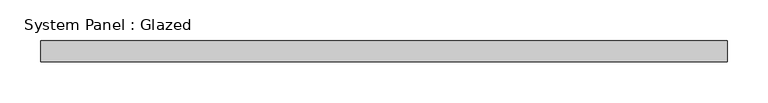
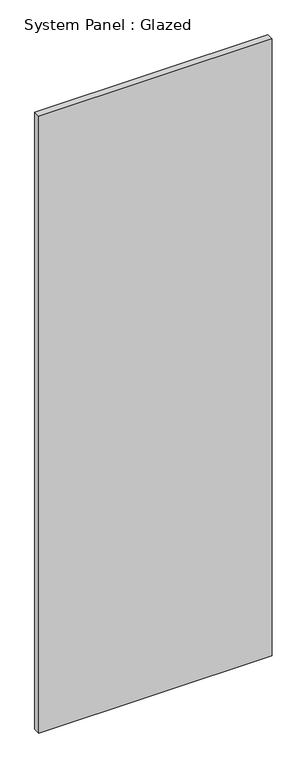
"""IFC4 building model written with IfcOpenShell, lengths in millimetres: plate geometry, System Panel : Glazed."""

from ifc_helpers import new_model, si_unit, origin, origin_with_axes, place, context, project, spatial, polyline, outline, extrude, source, transform, mapped, element, save


def system_panel_glazed_51086eaf(model_context):
    return source(origin(), model_context, "Body", "SweptSolid", [
        extrude(outline(polyline([(419.1, 19.05), (-419.1, 19.05), (-419.1, 44.45), (419.1, 44.45), (419.1, 19.05)])), origin_with_axes(), (0.0, 0.0, 1.0), 2343.15),
    ])


if __name__ == "__main__":
    model = new_model("IFC4")
    model_context = context("Model", 3, world=origin())
    ifc_project = project(units=[si_unit("LENGTHUNIT", "METRE", prefix="MILLI")], contexts=[model_context])
    site = spatial("IfcSite", under=ifc_project)
    building = spatial("IfcBuilding", under=site)
    placement = place(None, origin())
    system_panel_glazed_shape = system_panel_glazed_51086eaf(model_context)
    element("IfcPlate", 1, ObjectType="System Panel : Glazed", at=placement, inside=building, context=model_context, shape_type="MappedRepresentation", body=[
        mapped(system_panel_glazed_shape, transform((0.0, 0.0, 0.0), x_axis=(1.0, 0.0, 0.0), y_axis=(0.0, 1.0, 0.0), z_axis=(0.0, 0.0, 1.0))),
    ])
    save(model, "model.ifc")

# Revit data of these elements
# Type "System Panel : Glazed"
#   Construction Type Id = "GSP4R"
#   Analytic Construction = "1/8 in Pilkington single glazing"
#   Visual Light Transmittance = 0.9
#   Solar Heat Gain Coefficient = 0.86
#   Heat Transfer Coefficient (U) = 1.18115 BTU/(h·ft²·°F)
#   Define Thermal Properties by = 1
# Element 1 (IfcPlate, "System Panel : Glazed")
#   Materials on its faces: "glass panel 223"
# Materials
#   "glass panel 223": class "Generic", colour RGB 120 120 120, transparency 0, Cost = 0
